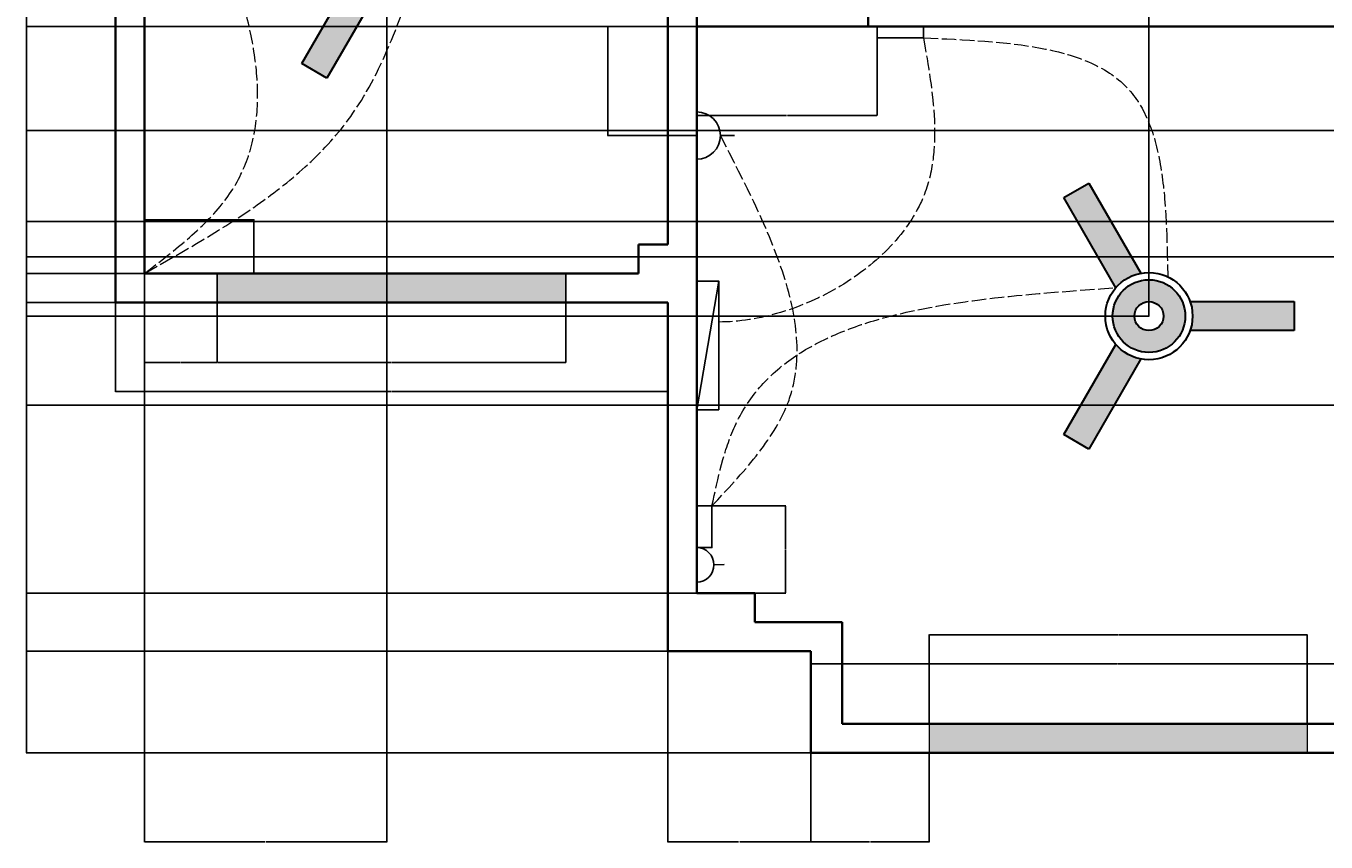
# Model space of a CAD drawing. Units: inches. Extents: x 2034 to 3646, y 962 to 2549.
# Tile 1 of 4: x 2034 to 3108, y 962 to 1636. Entities that reach past the tile are written whole.
import ezdxf

# ---------------------------------------------------------------- set-up
doc = ezdxf.new("R2010")
doc.units = ezdxf.units.IN
doc.linetypes.add('ACAD_ISO02W100', pattern=[15, 12, -3])
for name, color, linetype, lineweight in [('A-ANNO-DIMS', 2, 'Continuous', 18), ('A-GLAZ', 250, 'Continuous', 18), ('E-EQPM-FANS', 7, 'Continuous', 30), ('E-LITE-CTRL', 7, 'Continuous', 25), ('E-LITE-FIXT', 7, 'Continuous', 25), ('E-POWR-DEVC', 7, 'Continuous', 25)]:
    doc.layers.add(name, color=color, linetype=linetype, lineweight=lineweight)
for name, color, linetype, lineweight, true_color in [('A-GLAZ-PATT', 18, 'Continuous', 13, 0x000000), ('A-WALL', 203, 'Continuous', 35, 0xa780c2), ('E-LITE-WIRE', 103, 'ACAD_ISO02W100', 18, 0x6dc08b)]:
    doc.layers.add(name, color=color, linetype=linetype, lineweight=lineweight, true_color=true_color)
doc.styles.get("Standard").update_dxf_attribs({"font": 'arial.ttf'})
doc.dimstyles.get("Standard").update_dxf_attribs({"dimtxt": 0.18, "dimasz": 0.18, "dimexe": 0.18, "dimexo": 0.0625, "dimgap": 0.09, "dimtad": 0, "dimtih": 1, "dimtoh": 1, "dimdec": 4, "dimzin": 0, "dimdsep": 46, "dimtxsty": 'Standard', "dimcen": 0.09, "dimadec": 0, "dimazin": 0, "dimtfac": 1, "dimtdec": 4, "dimtofl": 0, "dimtmove": 0, "dimatfit": 3, "dimfxl": 1, "dimtolj": 1, "dimtzin": 0, "dimarcsym": 0})

# ---------------------------------------------------------------- blocks, each defined once
blk = doc.blocks.new('CEILING-FAN-3-BLADE')
h = blk.add_hatch(color=256)
h.dxf.hatch_style = 1
h.paths.add_polyline_path([(-49.6, 109.9), (-70.4, 97.9), (-27.4, 23.4, -0.171573), (-6.6, 35.4)])
h = blk.add_hatch(color=256)
h.dxf.hatch_style = 1
h.paths.add_polyline_path([(-30, 0, 1), (30, 0, 1)])
h.paths.add_polyline_path([(12, 0, -1), (-12, 0, -1)], flags=16)
h = blk.add_hatch(color=256)
h.dxf.hatch_style = 1
h.paths.add_polyline_path([(120, 12), (33.9, 12, -0.085164), (36, 0, -0.085164), (33.9, -12), (120, -12)])
h = blk.add_hatch(color=256)
h.dxf.hatch_style = 1
h.paths.add_polyline_path([(-6.6, -35.4, -0.171573), (-27.4, -23.4), (-70.4, -97.9), (-49.6, -109.9)])
for p, q in [((-70.4, 97.9), (-49.6, 109.9)), ((-49.6, 109.9), (-6.6, 35.4)), ((-27.4, 23.4), (-70.4, 97.9)), ((33.9, 12), (120, 12)), ((120, 12), (120, -12)), ((120, -12), (33.9, -12)), ((-70.4, -97.9), (-27.4, -23.4)), ((-6.6, -35.4), (-49.6, -109.9)), ((-49.6, -109.9), (-70.4, -97.9))]:
    blk.add_line(p, q)
for radius in [36, 30, 12]:
    blk.add_circle((0, 0), radius)
blk = doc.blocks.new('*D5')
at = {"layer": 'A-ANNO-DIMS', "color": 0, "lineweight": -2, "transparency": 16777216}
for p, q in [((2108.1, 2475.6), (2034.6, 2475.6)), ((2034.7, 2475.5), (2034.7, 1755.8)), ((2034.7, 1035.8), (2034.7, 1755.5)), ((2682.3, 1035.6), (2034.6, 1035.6))]:
    blk.add_line(p, q, dxfattribs=at)
at = {"layer": 'A-ANNO-DIMS', "color": 0, "transparency": 16777216}
for points in [[(2034.7, 2475.5), (2034.8, 2475.5), (2034.7, 2475.6)], [(2034.7, 1035.8), (2034.8, 1035.8), (2034.7, 1035.6)]]:
    blk.add_solid(points, dxfattribs=at)
at = {"layer": 'Defpoints', "color": 0, "transparency": 16777216}
for p in [(2034.7, 2475.6), (2108.2, 2475.6), (2682.3, 1035.6)]:
    blk.add_point(p, dxfattribs=at)
at = {"layer": 'A-ANNO-DIMS', "color": 0, "transparency": 16777216, "insert": (2034.7, 1755.6), "char_height": 0.18, "attachment_point": 5}
blk.add_mtext('\\A1;1440', dxfattribs=at)
blk = doc.blocks.new('*D6')
at = {"layer": 'A-ANNO-DIMS', "color": 0, "lineweight": -2, "transparency": 16777216}
for p, q in [((2108.2, 1407.6), (2108.2, 1334)), ((2564.2, 1407.6), (2564.2, 1334)), ((2108.4, 1334.2), (2335.9, 1334.2)), ((2564, 1334.2), (2336.5, 1334.2))]:
    blk.add_line(p, q, dxfattribs=at)
at = {"layer": 'A-ANNO-DIMS', "color": 0, "transparency": 16777216}
for points in [[(2108.4, 1334.2), (2108.4, 1334.2), (2108.2, 1334.2)], [(2564, 1334.2), (2564, 1334.2), (2564.2, 1334.2)]]:
    blk.add_solid(points, dxfattribs=at)
at = {"layer": 'Defpoints', "color": 0, "transparency": 16777216}
for p in [(2108.2, 1407.6), (2564.2, 1407.6), (2108.2, 1334.2)]:
    blk.add_point(p, dxfattribs=at)
at = {"layer": 'A-ANNO-DIMS', "color": 0, "transparency": 16777216, "insert": (2336.2, 1334.2), "char_height": 0.18, "attachment_point": 5}
blk.add_mtext('\\A1;456', dxfattribs=at)
blk = doc.blocks.new('*D7')
at = {"layer": 'A-ANNO-DIMS', "color": 0, "lineweight": -2, "transparency": 16777216}
for p, q in [((2564.2, 1119.6), (2564.2, 962)), ((2682.3, 1119.6), (2682.3, 962)), ((2564.4, 962.2), (2622.8, 962.2)), ((2682.1, 962.2), (2623.7, 962.2))]:
    blk.add_line(p, q, dxfattribs=at)
at = {"layer": 'A-ANNO-DIMS', "color": 0, "transparency": 16777216}
for points in [[(2564.4, 962.2), (2564.4, 962.2), (2564.2, 962.2)], [(2682.1, 962.2), (2682.1, 962.2), (2682.3, 962.2)]]:
    blk.add_solid(points, dxfattribs=at)
at = {"layer": 'Defpoints', "color": 0, "transparency": 16777216}
for p in [(2564.2, 1119.6), (2682.3, 1119.6), (2682.3, 962.2)]:
    blk.add_point(p, dxfattribs=at)
at = {"layer": 'A-ANNO-DIMS', "color": 0, "transparency": 16777216, "insert": (2623.3, 962.2), "char_height": 0.18, "attachment_point": 5}
blk.add_mtext('\\A1;118.12', dxfattribs=at)
blk = doc.blocks.new('*D8')
at = {"layer": 'A-ANNO-DIMS', "color": 0, "lineweight": -2, "transparency": 16777216}
for p, q in [((2682.3, 1035.7), (2682.3, 1109.3)), ((2682.5, 1109.1), (2935.5, 1109.1)), ((3189.4, 1109.1), (2936.3, 1109.1)), ((3189.6, 1035.7), (3189.6, 1109.3))]:
    blk.add_line(p, q, dxfattribs=at)
at = {"layer": 'A-ANNO-DIMS', "color": 0, "transparency": 16777216}
for points in [[(2682.5, 1109.1), (2682.5, 1109.1), (2682.3, 1109.1)], [(3189.4, 1109.1), (3189.4, 1109.1), (3189.6, 1109.1)]]:
    blk.add_solid(points, dxfattribs=at)
at = {"layer": 'Defpoints', "color": 0, "transparency": 16777216}
for p in [(3189.6, 1109.1), (2682.3, 1035.6), (3189.6, 1035.6)]:
    blk.add_point(p, dxfattribs=at)
at = {"layer": 'A-ANNO-DIMS', "color": 0, "transparency": 16777216, "insert": (2935.9, 1109.1), "char_height": 0.18, "attachment_point": 5}
blk.add_mtext('\\A1;507.2', dxfattribs=at)
blk = doc.blocks.new('*D9')
at = {"layer": 'A-ANNO-DIMS', "color": 0, "lineweight": -2, "transparency": 16777216}
for p, q in [((2564.1, 1407.6), (2034.6, 1407.6)), ((2034.7, 1407.5), (2034.7, 1263.8)), ((2034.7, 1119.8), (2034.7, 1263.5)), ((2564.1, 1119.6), (2034.6, 1119.6))]:
    blk.add_line(p, q, dxfattribs=at)
at = {"layer": 'A-ANNO-DIMS', "color": 0, "transparency": 16777216}
for points in [[(2034.7, 1407.5), (2034.8, 1407.5), (2034.7, 1407.6)], [(2034.7, 1119.8), (2034.8, 1119.8), (2034.7, 1119.6)]]:
    blk.add_solid(points, dxfattribs=at)
at = {"layer": 'Defpoints', "color": 0, "transparency": 16777216}
for p in [(2034.7, 1407.6), (2564.2, 1407.6), (2564.2, 1119.6)]:
    blk.add_point(p, dxfattribs=at)
at = {"layer": 'A-ANNO-DIMS', "color": 0, "transparency": 16777216, "insert": (2034.7, 1263.6), "char_height": 0.18, "attachment_point": 5}
blk.add_mtext('\\A1;288', dxfattribs=at)
blk = doc.blocks.new('*D10')
at = {"layer": 'A-ANNO-DIMS', "color": 0, "lineweight": -2, "transparency": 16777216}
for p, q in [((2682.3, 1119.6), (2034.6, 1119.6)), ((2034.7, 1119.5), (2034.7, 1077.8)), ((2034.7, 1035.8), (2034.7, 1077.5)), ((2682.3, 1035.6), (2034.6, 1035.6))]:
    blk.add_line(p, q, dxfattribs=at)
at = {"layer": 'A-ANNO-DIMS', "color": 0, "transparency": 16777216}
for points in [[(2034.7, 1119.5), (2034.8, 1119.5), (2034.7, 1119.6)], [(2034.7, 1035.8), (2034.8, 1035.8), (2034.7, 1035.6)]]:
    blk.add_solid(points, dxfattribs=at)
at = {"layer": 'Defpoints', "color": 0, "transparency": 16777216}
for p in [(2034.7, 1119.6), (2682.3, 1119.6), (2682.3, 1035.6)]:
    blk.add_point(p, dxfattribs=at)
at = {"layer": 'A-ANNO-DIMS', "color": 0, "transparency": 16777216, "insert": (2034.7, 1077.6), "char_height": 0.18, "attachment_point": 5}
blk.add_mtext('\\A1;84', dxfattribs=at)
blk = doc.blocks.new('*D16')
at = {"layer": 'A-ANNO-DIMS', "color": 0, "lineweight": -2, "transparency": 16777216}
for p, q in [((2588.2, 1635.7), (2588.2, 2549.3)), ((2588.4, 2549.1), (2935.9, 2549.1)), ((3284, 2549.1), (2936.5, 2549.1)), ((3284.2, 1635.7), (3284.2, 2549.3))]:
    blk.add_line(p, q, dxfattribs=at)
at = {"layer": 'A-ANNO-DIMS', "color": 0, "transparency": 16777216}
for points in [[(2588.4, 2549.1), (2588.4, 2549.1), (2588.2, 2549.1)], [(3284, 2549.1), (3284, 2549.1), (3284.2, 2549.1)]]:
    blk.add_solid(points, dxfattribs=at)
at = {"layer": 'Defpoints', "color": 0, "transparency": 16777216}
for p in [(3284.2, 2549.1), (2588.2, 1635.6), (3284.2, 1635.6)]:
    blk.add_point(p, dxfattribs=at)
at = {"layer": 'A-ANNO-DIMS', "color": 0, "transparency": 16777216, "insert": (2936.2, 2549.1), "char_height": 0.18, "attachment_point": 5}
blk.add_mtext('\\A1;696', dxfattribs=at)
blk = doc.blocks.new('*D17')
at = {"layer": 'A-ANNO-DIMS', "color": 0, "lineweight": -2, "transparency": 16777216}
for p, q in [((2588.1, 1635.6), (2034.6, 1635.6)), ((2034.7, 1635.5), (2034.7, 1401.8)), ((2034.7, 1167.8), (2034.7, 1401.5)), ((2588.1, 1167.6), (2034.6, 1167.6))]:
    blk.add_line(p, q, dxfattribs=at)
at = {"layer": 'A-ANNO-DIMS', "color": 0, "transparency": 16777216}
for points in [[(2034.7, 1635.5), (2034.8, 1635.5), (2034.7, 1635.6)], [(2034.7, 1167.8), (2034.8, 1167.8), (2034.7, 1167.6)]]:
    blk.add_solid(points, dxfattribs=at)
at = {"layer": 'Defpoints', "color": 0, "transparency": 16777216}
for p in [(2034.7, 1635.6), (2588.2, 1635.6), (2588.2, 1167.6)]:
    blk.add_point(p, dxfattribs=at)
at = {"layer": 'A-ANNO-DIMS', "color": 0, "transparency": 16777216, "insert": (2034.7, 1401.6), "char_height": 0.18, "attachment_point": 5}
blk.add_mtext('\\A1;468', dxfattribs=at)
blk = doc.blocks.new('*D30')
at = {"layer": 'A-ANNO-DIMS', "color": 0, "lineweight": -2, "transparency": 16777216}
for p, q in [((2332.4, 1702.8), (2332.4, 962)), ((2132.2, 1431.6), (2132.2, 962)), ((2132.4, 962.2), (2231.9, 962.2)), ((2332.3, 962.2), (2232.8, 962.2))]:
    blk.add_line(p, q, dxfattribs=at)
at = {"layer": 'A-ANNO-DIMS', "color": 0, "transparency": 16777216}
for points in [[(2132.4, 962.2), (2132.4, 962.2), (2132.2, 962.2)], [(2332.3, 962.2), (2332.3, 962.2), (2332.4, 962.2)]]:
    blk.add_solid(points, dxfattribs=at)
at = {"layer": 'Defpoints', "color": 0, "transparency": 16777216}
for p in [(2332.4, 1702.9), (2132.2, 1431.6), (2332.4, 962.2)]:
    blk.add_point(p, dxfattribs=at)
at = {"layer": 'A-ANNO-DIMS', "color": 0, "transparency": 16777216, "insert": (2232.3, 962.2), "char_height": 0.18, "attachment_point": 5}
blk.add_mtext('\\A1;200.24', dxfattribs=at)
blk = doc.blocks.new('*D31')
at = {"layer": 'A-ANNO-DIMS', "color": 0, "lineweight": -2, "transparency": 16777216}
for p, q in [((2332.4, 1702.9), (2034.6, 1702.9)), ((2034.7, 1702.7), (2034.7, 1567.4)), ((2034.7, 1431.8), (2034.7, 1567.1)), ((2132.1, 1431.6), (2034.6, 1431.6))]:
    blk.add_line(p, q, dxfattribs=at)
at = {"layer": 'A-ANNO-DIMS', "color": 0, "transparency": 16777216}
for points in [[(2034.7, 1702.7), (2034.8, 1702.7), (2034.7, 1702.9)], [(2034.7, 1431.8), (2034.8, 1431.8), (2034.7, 1431.6)]]:
    blk.add_solid(points, dxfattribs=at)
at = {"layer": 'Defpoints', "color": 0, "transparency": 16777216}
for p in [(2034.7, 1702.9), (2332.4, 1702.9), (2132.2, 1431.6)]:
    blk.add_point(p, dxfattribs=at)
at = {"layer": 'A-ANNO-DIMS', "color": 0, "transparency": 16777216, "insert": (2034.7, 1567.3), "char_height": 0.18, "attachment_point": 5}
blk.add_mtext('\\A1;271.24', dxfattribs=at)
blk = doc.blocks.new('*D33')
at = {"layer": 'A-ANNO-DIMS', "color": 0, "lineweight": -2, "transparency": 16777216}
for p, q in [((2961.6, 1396.5), (2961.6, 2549.3)), ((2961.8, 2549.1), (3122.5, 2549.1)), ((3284, 2549.1), (3123.3, 2549.1)), ((3284.2, 1305), (3284.2, 2549.3))]:
    blk.add_line(p, q, dxfattribs=at)
at = {"layer": 'A-ANNO-DIMS', "color": 0, "transparency": 16777216}
for points in [[(2961.8, 2549.1), (2961.8, 2549.1), (2961.6, 2549.1)], [(3284, 2549.1), (3284, 2549.1), (3284.2, 2549.1)]]:
    blk.add_solid(points, dxfattribs=at)
at = {"layer": 'Defpoints', "color": 0, "transparency": 16777216}
for p in [(3284.2, 2549.1), (2961.6, 1396.4), (3284.2, 1304.9)]:
    blk.add_point(p, dxfattribs=at)
at = {"layer": 'A-ANNO-DIMS', "color": 0, "transparency": 16777216, "insert": (3122.9, 2549.1), "char_height": 0.18, "attachment_point": 5}
blk.add_mtext('\\A1;322.6', dxfattribs=at)
blk = doc.blocks.new('*D34')
at = {"layer": 'A-ANNO-DIMS', "color": 0, "lineweight": -2, "transparency": 16777216}
for p, q in [((2737.1, 1635.6), (2034.6, 1635.6)), ((2034.7, 1635.5), (2034.7, 1516.2)), ((2034.7, 1396.6), (2034.7, 1515.9)), ((2961.5, 1396.4), (2034.6, 1396.4))]:
    blk.add_line(p, q, dxfattribs=at)
at = {"layer": 'A-ANNO-DIMS', "color": 0, "transparency": 16777216}
for points in [[(2034.7, 1635.5), (2034.8, 1635.5), (2034.7, 1635.6)], [(2034.7, 1396.6), (2034.8, 1396.6), (2034.7, 1396.4)]]:
    blk.add_solid(points, dxfattribs=at)
at = {"layer": 'Defpoints', "color": 0, "transparency": 16777216}
for p in [(2034.7, 1635.6), (2737.2, 1635.6), (2961.6, 1396.4)]:
    blk.add_point(p, dxfattribs=at)
at = {"layer": 'A-ANNO-DIMS', "color": 0, "transparency": 16777216, "insert": (2034.7, 1516), "char_height": 0.18, "attachment_point": 5}
blk.add_mtext('\\A1;239.2', dxfattribs=at)
blk = doc.blocks.new('*D35')
at = {"layer": 'A-ANNO-DIMS', "color": 0, "lineweight": -2, "transparency": 16777216}
for p, q in [((2132.2, 1431.6), (2132.2, 1358)), ((2192.2, 1431.6), (2192.2, 1358)), ((2132.4, 1358.2), (2162, 1358.2)), ((2192, 1358.2), (2162.4, 1358.2))]:
    blk.add_line(p, q, dxfattribs=at)
at = {"layer": 'A-ANNO-DIMS', "color": 0, "transparency": 16777216}
for points in [[(2132.4, 1358.2), (2132.4, 1358.2), (2132.2, 1358.2)], [(2192, 1358.2), (2192, 1358.2), (2192.2, 1358.2)]]:
    blk.add_solid(points, dxfattribs=at)
at = {"layer": 'Defpoints', "color": 0, "transparency": 16777216}
for p in [(2132.2, 1431.6), (2192.2, 1431.6), (2132.2, 1358.2)]:
    blk.add_point(p, dxfattribs=at)
at = {"layer": 'A-ANNO-DIMS', "color": 0, "transparency": 16777216, "insert": (2162.2, 1358.2), "char_height": 0.18, "attachment_point": 5}
blk.add_mtext('\\A1;60', dxfattribs=at)
blk = doc.blocks.new('*D36')
at = {"layer": 'A-ANNO-DIMS', "color": 0, "lineweight": -2, "transparency": 16777216}
for p, q in [((2192.2, 1431.6), (2192.2, 1358)), ((2480.2, 1431.6), (2480.2, 1358)), ((2192.4, 1358.2), (2335.9, 1358.2)), ((2480, 1358.2), (2336.5, 1358.2))]:
    blk.add_line(p, q, dxfattribs=at)
at = {"layer": 'A-ANNO-DIMS', "color": 0, "transparency": 16777216}
for points in [[(2192.4, 1358.2), (2192.4, 1358.2), (2192.2, 1358.2)], [(2480, 1358.2), (2480, 1358.2), (2480.2, 1358.2)]]:
    blk.add_solid(points, dxfattribs=at)
at = {"layer": 'Defpoints', "color": 0, "transparency": 16777216}
for p in [(2192.2, 1431.6), (2480.2, 1431.6), (2192.2, 1358.2)]:
    blk.add_point(p, dxfattribs=at)
at = {"layer": 'A-ANNO-DIMS', "color": 0, "transparency": 16777216, "insert": (2336.2, 1358.2), "char_height": 0.18, "attachment_point": 5}
blk.add_mtext('\\A1;288', dxfattribs=at)
blk = doc.blocks.new('*D37')
at = {"layer": 'A-ANNO-DIMS', "color": 0, "lineweight": -2, "transparency": 16777216}
for p, q in [((2682.3, 1035.6), (2682.3, 962)), ((2780.2, 1035.6), (2780.2, 962)), ((2682.5, 962.2), (2730.9, 962.2)), ((2780, 962.2), (2731.7, 962.2))]:
    blk.add_line(p, q, dxfattribs=at)
at = {"layer": 'A-ANNO-DIMS', "color": 0, "transparency": 16777216}
for points in [[(2682.5, 962.2), (2682.5, 962.2), (2682.3, 962.2)], [(2780, 962.2), (2780, 962.2), (2780.2, 962.2)]]:
    blk.add_solid(points, dxfattribs=at)
at = {"layer": 'Defpoints', "color": 0, "transparency": 16777216}
for p in [(2682.3, 1035.6), (2780.2, 1035.6), (2780.2, 962.2)]:
    blk.add_point(p, dxfattribs=at)
at = {"layer": 'A-ANNO-DIMS', "color": 0, "transparency": 16777216, "insert": (2731.3, 962.2), "char_height": 0.18, "attachment_point": 5}
blk.add_mtext('\\A1;97.88', dxfattribs=at)
blk = doc.blocks.new('*D38')
at = {"layer": 'A-ANNO-DIMS', "color": 0, "lineweight": -2, "transparency": 16777216}
for p, q in [((2780.2, 1059.7), (2780.2, 1133.3)), ((2780.4, 1133.1), (2935.9, 1133.1)), ((3092, 1133.1), (2936.5, 1133.1)), ((3092.2, 1059.7), (3092.2, 1133.3))]:
    blk.add_line(p, q, dxfattribs=at)
at = {"layer": 'A-ANNO-DIMS', "color": 0, "transparency": 16777216}
for points in [[(2780.4, 1133.1), (2780.4, 1133.1), (2780.2, 1133.1)], [(3092, 1133.1), (3092, 1133.1), (3092.2, 1133.1)]]:
    blk.add_solid(points, dxfattribs=at)
at = {"layer": 'Defpoints', "color": 0, "transparency": 16777216}
for p in [(3092.2, 1133.1), (2780.2, 1059.6), (3092.2, 1059.6)]:
    blk.add_point(p, dxfattribs=at)
at = {"layer": 'A-ANNO-DIMS', "color": 0, "transparency": 16777216, "insert": (2936.2, 1133.1), "char_height": 0.18, "attachment_point": 5}
blk.add_mtext('\\A1;312', dxfattribs=at)
blk = doc.blocks.new('*D49')
at = {"layer": 'A-ANNO-DIMS', "color": 0, "lineweight": -2, "transparency": 16777216}
for p, q in [((3392.3, 1474.6), (2034.6, 1474.6)), ((2034.7, 1474.4), (2034.7, 1398.9)), ((2034.7, 1323), (2034.7, 1398.5)), ((3392.3, 1322.8), (2034.6, 1322.8))]:
    blk.add_line(p, q, dxfattribs=at)
at = {"layer": 'A-ANNO-DIMS', "color": 0, "transparency": 16777216}
for points in [[(2034.7, 1474.4), (2034.8, 1474.4), (2034.7, 1474.6)], [(2034.7, 1323), (2034.8, 1323), (2034.7, 1322.8)]]:
    blk.add_solid(points, dxfattribs=at)
at = {"layer": 'Defpoints', "color": 0, "transparency": 16777216}
for p in [(2034.7, 1474.6), (3392.3, 1474.6), (3392.3, 1322.8)]:
    blk.add_point(p, dxfattribs=at)
at = {"layer": 'A-ANNO-DIMS', "color": 0, "transparency": 16777216, "insert": (2034.7, 1398.7), "char_height": 0.18, "attachment_point": 5}
blk.add_mtext('\\A1;151.76', dxfattribs=at)
blk = doc.blocks.new('*D52')
at = {"layer": 'A-ANNO-DIMS', "color": 0, "lineweight": -2, "transparency": 16777216}
for p, q in [((3284.1, 1549.7), (2034.6, 1549.7)), ((2034.7, 1549.5), (2034.7, 1497.7)), ((2034.7, 1445.5), (2034.7, 1497.3)), ((3284.1, 1445.3), (2034.6, 1445.3))]:
    blk.add_line(p, q, dxfattribs=at)
at = {"layer": 'A-ANNO-DIMS', "color": 0, "transparency": 16777216}
for points in [[(2034.7, 1549.5), (2034.8, 1549.5), (2034.7, 1549.7)], [(2034.7, 1445.5), (2034.8, 1445.5), (2034.7, 1445.3)]]:
    blk.add_solid(points, dxfattribs=at)
at = {"layer": 'Defpoints', "color": 0, "transparency": 16777216}
for p in [(2034.7, 1549.7), (3284.2, 1549.7), (3284.2, 1445.3)]:
    blk.add_point(p, dxfattribs=at)
at = {"layer": 'A-ANNO-DIMS', "color": 0, "transparency": 16777216, "insert": (2034.7, 1497.5), "char_height": 0.18, "attachment_point": 5}
blk.add_mtext('\\A1;104.39', dxfattribs=at)
blk = doc.blocks.new('*D54')
at = {"layer": 'A-ANNO-DIMS', "color": 0, "lineweight": -2, "transparency": 16777216}
for p, q in [((2588.2, 1635.6), (2588.2, 1562)), ((2737.2, 1635.6), (2737.2, 1562)), ((2588.4, 1562.2), (2662.2, 1562.2)), ((2737, 1562.2), (2663.1, 1562.2))]:
    blk.add_line(p, q, dxfattribs=at)
at = {"layer": 'A-ANNO-DIMS', "color": 0, "transparency": 16777216}
for points in [[(2588.4, 1562.2), (2588.4, 1562.2), (2588.2, 1562.2)], [(2737, 1562.2), (2737, 1562.2), (2737.2, 1562.2)]]:
    blk.add_solid(points, dxfattribs=at)
at = {"layer": 'Defpoints', "color": 0, "transparency": 16777216}
for p in [(2588.2, 1635.6), (2737.2, 1635.6), (2588.2, 1562.2)]:
    blk.add_point(p, dxfattribs=at)
at = {"layer": 'A-ANNO-DIMS', "color": 0, "transparency": 16777216, "insert": (2662.7, 1562.2), "char_height": 0.18, "attachment_point": 5}
blk.add_mtext('\\A1;148.97', dxfattribs=at)
blk = doc.blocks.new('*D58')
at = {"layer": 'A-ANNO-DIMS', "color": 0, "lineweight": -2, "transparency": 16777216}
for p, q in [((2588.1, 1635.6), (2514.6, 1635.6)), ((2514.7, 1635.5), (2514.7, 1590.8)), ((2514.7, 1545.7), (2514.7, 1590.4)), ((2588.1, 1545.5), (2514.6, 1545.5))]:
    blk.add_line(p, q, dxfattribs=at)
at = {"layer": 'A-ANNO-DIMS', "color": 0, "transparency": 16777216}
for points in [[(2514.7, 1635.5), (2514.8, 1635.5), (2514.7, 1635.6)], [(2514.7, 1545.7), (2514.8, 1545.7), (2514.7, 1545.5)]]:
    blk.add_solid(points, dxfattribs=at)
at = {"layer": 'Defpoints', "color": 0, "transparency": 16777216}
for p in [(2514.7, 1635.6), (2588.2, 1635.6), (2588.2, 1545.5)]:
    blk.add_point(p, dxfattribs=at)
at = {"layer": 'A-ANNO-DIMS', "color": 0, "transparency": 16777216, "insert": (2514.7, 1590.6), "char_height": 0.18, "attachment_point": 5}
blk.add_mtext('\\A1;90.1', dxfattribs=at)
blk = doc.blocks.new('*D60')
at = {"layer": 'A-ANNO-DIMS', "color": 0, "lineweight": -2, "transparency": 16777216}
for p, q in [((2588.3, 1239.6), (2661.8, 1239.6)), ((2661.6, 1239.4), (2661.6, 1203.8)), ((2661.6, 1167.8), (2661.6, 1203.4)), ((2588.3, 1167.6), (2661.8, 1167.6))]:
    blk.add_line(p, q, dxfattribs=at)
at = {"layer": 'A-ANNO-DIMS', "color": 0, "transparency": 16777216}
for points in [[(2661.6, 1239.4), (2661.7, 1239.4), (2661.6, 1239.6)], [(2661.6, 1167.8), (2661.7, 1167.8), (2661.6, 1167.6)]]:
    blk.add_solid(points, dxfattribs=at)
at = {"layer": 'Defpoints', "color": 0, "transparency": 16777216}
for p in [(2588.2, 1239.6), (2588.2, 1167.6), (2661.6, 1167.6)]:
    blk.add_point(p, dxfattribs=at)
at = {"layer": 'A-ANNO-DIMS', "color": 0, "transparency": 16777216, "insert": (2661.6, 1203.6), "char_height": 0.18, "attachment_point": 5}
blk.add_mtext('\\A1;71.98', dxfattribs=at)
blk = doc.blocks.new('*D64')
at = {"layer": 'A-ANNO-DIMS', "color": 0, "lineweight": -2, "transparency": 16777216}
for p, q in [((2904, 1396.4), (2925.4, 1396.4)), ((2961.5, 1396.4), (2961.7, 1396.4)), ((2961.6, 1396.3), (2961.6, 1396.5))]:
    blk.add_line(p, q, dxfattribs=at)
at = {"layer": 'A-ANNO-DIMS', "color": 0, "transparency": 16777216}
blk.add_solid([(2925.4, 1396.5), (2925.4, 1396.4), (2925.6, 1396.4)], dxfattribs=at)
at = {"layer": 'Defpoints', "color": 0, "transparency": 16777216}
for p in [(2925.6, 1396.4), (2997.6, 1396.4)]:
    blk.add_point(p, dxfattribs=at)
at = {"layer": 'A-ANNO-DIMS', "color": 0, "transparency": 16777216, "insert": (2903.5, 1396.4), "char_height": 0.18, "attachment_point": 5}
blk.add_mtext('\\A1;4X ∅72', dxfattribs=at)
blk = doc.blocks.new('*D72')
at = {"layer": 'A-ANNO-DIMS', "color": 0, "lineweight": -2, "transparency": 16777216}
for p, q in [((2588.1, 1545.5), (2588.3, 1545.5)), ((2588.2, 1545.4), (2588.2, 1545.6)), ((2619.4, 1545.5), (2607.9, 1545.5))]:
    blk.add_line(p, q, dxfattribs=at)
at = {"layer": 'A-ANNO-DIMS', "color": 0, "transparency": 16777216}
blk.add_solid([(2607.9, 1545.6), (2607.9, 1545.5), (2607.7, 1545.5)], dxfattribs=at)
at = {"layer": 'Defpoints', "color": 0, "transparency": 16777216}
for p in [(2588.2, 1545.5), (2607.7, 1545.5)]:
    blk.add_point(p, dxfattribs=at)
at = {"layer": 'A-ANNO-DIMS', "color": 0, "transparency": 16777216, "insert": (2620, 1545.5), "char_height": 0.18, "attachment_point": 5}
blk.add_mtext('\\A1;R19.526', dxfattribs=at)
blk = doc.blocks.new('*D78')
at = {"layer": 'A-ANNO-DIMS', "color": 0, "lineweight": -2, "transparency": 16777216}
for p, q in [((2588.1, 1190.9), (2588.3, 1190.9)), ((2588.2, 1190.9), (2588.2, 1191)), ((2610.9, 1191.2), (2602.6, 1191.1))]:
    blk.add_line(p, q, dxfattribs=at)
at = {"layer": 'A-ANNO-DIMS', "color": 0, "transparency": 16777216}
blk.add_solid([(2602.6, 1191.1), (2602.6, 1191.1), (2602.4, 1191.1)], dxfattribs=at)
at = {"layer": 'Defpoints', "color": 0, "transparency": 16777216}
for p in [(2588.2, 1190.9), (2602.4, 1191.1)]:
    blk.add_point(p, dxfattribs=at)
at = {"layer": 'A-ANNO-DIMS', "color": 0, "transparency": 16777216, "insert": (2611.4, 1191.2), "char_height": 0.18, "attachment_point": 5}
blk.add_mtext('\\A1;R14.22', dxfattribs=at)

msp = doc.modelspace()

# ---------------------------------------------------------------- hatches: boundary and pattern name
at = {"layer": 'A-GLAZ-PATT'}
h = msp.add_hatch(color=256, dxfattribs=at)
h.dxf.hatch_style = 1
h.paths.add_polyline_path([(2480.1976, 1431.6388), (2192.1976, 1431.6388), (2192.1976, 1407.6388), (2480.1976, 1407.6388)])
h = msp.add_hatch(color=256, dxfattribs=at)
h.dxf.hatch_style = 1
h.paths.add_polyline_path([(3092.1976, 1059.6388), (2780.1976, 1059.6388), (2780.1976, 1035.6388), (3092.1976, 1035.6388)])

# ---------------------------------------------------------------- linework, layer by layer
at = {"layer": 'A-GLAZ'}
for p, q in [((2192.1976, 1431.6388), (2192.1976, 1407.6388)), ((2192.1976, 1431.6388), (2480.1976, 1431.6388)), ((2480.1976, 1431.6388), (2480.1976, 1407.6388)), ((2192.1976, 1407.6388), (2480.1976, 1407.6388)), ((2780.1976, 1059.6388), (2780.1976, 1035.6388)), ((2780.1976, 1059.6388), (3092.1976, 1059.6388)), ((3092.1976, 1059.6388), (3092.1976, 1035.6388)), ((2780.1976, 1035.6388), (3092.1976, 1035.6388))]:
    msp.add_line(p, q, dxfattribs=at)
at = {"layer": 'A-WALL'}
for p, q in [((2588.1976, 1167.6388), (2588.1976, 1971.6388)), ((2132.1976, 1431.6388), (2132.1976, 1947.6388)), ((2564.1976, 1455.6388), (2564.1976, 1875.6388)), ((2729.8258, 1659.6388), (2729.8258, 1635.6388)), ((2588.1976, 1635.6388), (3284.1976, 1635.6388)), ((2540.1976, 1431.6388), (2540.1976, 1455.6388)), ((2540.1976, 1455.6388), (2564.1976, 1455.6388)), ((2132.1976, 1431.6388), (2540.1976, 1431.6388)), ((2132.1976, 1407.6388), (2108.1976, 1407.6388)), ((2132.1976, 1407.6388), (2564.1976, 1407.6388)), ((2564.1976, 1119.6388), (2564.1976, 1407.6388)), ((2636.1976, 1167.6388), (2588.1976, 1167.6388)), ((2636.1976, 1143.6388), (2636.1976, 1167.6388)), ((2708.1976, 1143.6388), (2636.1976, 1143.6388)), ((2708.1976, 1059.6388), (2708.1976, 1143.6388)), ((2682.3208, 1119.6388), (2564.1976, 1119.6388)), ((2682.3208, 1035.6388), (2682.3208, 1119.6388)), ((3164.1976, 1059.6388), (2708.1976, 1059.6388)), ((3189.5638, 1035.6388), (2682.3208, 1035.6388)), ((2706.3208, 1035.6388), (2682.3208, 1035.6388))]:
    msp.add_line(p, q, dxfattribs=at)
msp.add_lwpolyline([(2108.1976, 1407.6388), (2108.1976, 2475.6388), (3308.1976, 2475.6388)], dxfattribs=at)
at = {"layer": 'E-LITE-CTRL'}
for points in [[(2737.172, 1635.6388), (2775.458, 1635.6388), (2775.458, 1626.2502), (2737.172, 1626.2502)], [(2132.1976, 1431.6388), (2222.5717, 1431.6388), (2222.5717, 1476.0422), (2132.1976, 1476.0422)], [(2588.1976, 1205.1613), (2600.7258, 1205.1613), (2600.7258, 1239.6163), (2588.1976, 1239.6163)]]:
    msp.add_lwpolyline(points, close=True, dxfattribs=at)
at = {"layer": 'E-LITE-FIXT'}
msp.add_line((2606.4152, 1425.3903), (2588.1976, 1319.1329), dxfattribs=at)
msp.add_lwpolyline([(2588.1976, 1425.3903), (2606.4152, 1425.3903), (2606.4152, 1319.1329), (2588.1976, 1319.1329)], close=True, dxfattribs=at)
at = {"layer": 'E-LITE-WIRE'}
for points, knots in [([(2132.1976, 1431.6388), (2157.638, 1451.201), (2276.6339, 1542.7023), (2202.4164, 1700.7955), (2144.0659, 1825.0897)], [0, 0, 0, 0, 91.463199701, 427.814592014, 427.814592014, 427.814592014, 427.814592014]), ([(2132.1976, 1431.6388), (2198.2305, 1468.9918), (2306.37, 1530.1634), (2344.9098, 1645.8124), (2359.9161, 1690.843)], [0, 0, 0, 0, 217.156530493, 355.629044919, 355.629044919, 355.629044919, 355.629044919]), ([(2775.458, 1626.2502), (2783.4011, 1580.4234), (2803.3836, 1465.1371), (2672.4325, 1391.5072), (2606.2065, 1391.5305), (2606.1022, 1391.5306)], [0, 0, 0, 0, 130.887293215, 329.272351587, 329.58530176, 329.58530176, 329.58530176, 329.58530176]), ([(2775.458, 1626.2502), (2843.6443, 1623.2777), (2973.5056, 1617.6165), (2975.9452, 1489.6758), (2977.1038, 1428.9129)], [0, 0, 0, 0, 174.709563386, 332.73592807, 332.73592807, 332.73592807, 332.73592807]), ([(2600.7258, 1239.6163), (2626.1963, 1266.8392), (2707.0266, 1353.2306), (2648.0893, 1467.3625), (2607.7239, 1545.5301)], [0, 0, 0, 0, 105.060462832, 333.407204691, 333.407204691, 333.407204691, 333.407204691]), ([(2600.7258, 1239.6163), (2605.7381, 1262.7247), (2635.286, 1398.9506), (2798.6057, 1410.3546), (2934.221, 1419.8241)], [0, 0, 0, 0, 68.392765865, 403.180988759, 403.180988759, 403.180988759, 403.180988759])]:
    msp.add_open_spline(points, degree=3, knots=knots, dxfattribs=at)
at = {"layer": 'E-POWR-DEVC'}
for centre, radius in [((2588.1976, 1545.5301), 19.5263), ((2588.1976, 1190.9418), 14.2195)]:
    msp.add_arc(centre, radius, 270, 90, dxfattribs=at)

# ---------------------------------------------------------------- block references
at = {"layer": 'E-EQPM-FANS'}
for p in [(2332.4379, 1702.8825), (2961.5838, 1396.4302)]:
    msp.add_blockref('CEILING-FAN-3-BLADE', p, dxfattribs=at)

# ---------------------------------------------------------------- dimensions: what is measured, and where the dimension line sits
at = {"layer": 'A-ANNO-DIMS'}
for base, p1, p2, override, picture, middle in [((3284.1976, 2549.0888), (2588.1976, 1635.6388), (3284.1976, 1635.6388), {"dimdec": 0, "dimlfac": 1, "dimrnd": 0, "dimzin": 0, "dimdsep": 46, "dimlunit": 2}, '*D16', (2936.1976, 2549.0888)), ((3284.1976, 2549.0888), (2961.5838, 1396.4302), (3284.1976, 1304.9248), {"dimdec": 1, "dimlfac": 1, "dimrnd": 0, "dimzin": 0, "dimdsep": 46, "dimlunit": 2}, '*D33', (3122.8907, 2549.0888)), ((2332.4379, 962.1888), (2132.1976, 1431.6388), (2332.4379, 1702.8825), {"dimdec": 2, "dimlfac": 1, "dimrnd": 0, "dimzin": 0, "dimdsep": 46, "dimlunit": 2}, '*D30', (2232.3178, 962.1888)), ((3092.1976, 1133.0888), (2780.1976, 1059.6388), (3092.1976, 1059.6388), {"dimdec": 0, "dimlfac": 1, "dimrnd": 0, "dimzin": 0, "dimdsep": 46, "dimlunit": 2}, '*D38', (2936.1976, 1133.0888)), ((2682.3208, 962.1888), (2564.1976, 1119.6388), (2682.3208, 1119.6388), {"dimdec": 2, "dimlfac": 1, "dimrnd": 0, "dimzin": 0, "dimdsep": 46, "dimlunit": 2}, '*D7', (2623.2592, 962.1888)), ((3189.5638, 1109.0888), (2682.3208, 1035.6388), (3189.5638, 1035.6388), {"dimdec": 1, "dimlfac": 1, "dimrnd": 0, "dimzin": 0, "dimdsep": 46, "dimlunit": 2}, '*D8', (2935.9423, 1109.0888)), ((2780.1976, 962.1888), (2682.3208, 1035.6388), (2780.1976, 1035.6388), {"dimdec": 2, "dimlfac": 1, "dimrnd": 0, "dimzin": 0, "dimdsep": 46, "dimlunit": 2}, '*D37', (2731.2592, 962.1888))]:
    dim = msp.add_linear_dim(base=base, p1=p1, p2=p2, dimstyle='Standard', override=override, dxfattribs=at)
    dim.commit()
    dim.dimension.update_dxf_attribs({"geometry": picture, "text_midpoint": middle})
for base, p1, p2, angle, override, picture, middle in [((2034.7476, 2475.6388), (2682.3208, 1035.6388), (2108.1976, 2475.6388), 90, {"dimdec": 0, "dimlfac": 1, "dimrnd": 0, "dimzin": 0, "dimdsep": 46, "dimlunit": 2}, '*D5', (2034.7476, 1755.6388)), ((2034.7476, 1702.8825), (2132.1976, 1431.6388), (2332.4379, 1702.8825), 90, {"dimdec": 2, "dimlfac": 1, "dimrnd": 0, "dimzin": 0, "dimdsep": 46, "dimlunit": 2}, '*D31', (2034.7476, 1567.2606)), ((2034.7476, 1635.6388), (2961.5838, 1396.4302), (2737.172, 1635.6388), 90, {"dimdec": 1, "dimlfac": 1, "dimrnd": 0, "dimzin": 0, "dimdsep": 46, "dimlunit": 2}, '*D34', (2034.7476, 1516.0345)), ((2034.7476, 1635.6388), (2588.1976, 1167.6388), (2588.1976, 1635.6388), 90, {"dimdec": 0, "dimlfac": 1, "dimrnd": 0, "dimzin": 0, "dimdsep": 46, "dimlunit": 2}, '*D17', (2034.7476, 1401.6388)), ((2514.7476, 1635.6388), (2588.1976, 1545.5301), (2588.1976, 1635.6388), 90, {"dimdec": 1, "dimlfac": 1, "dimrnd": 0, "dimzin": 0, "dimdsep": 46, "dimlunit": 2}, '*D58', (2514.7476, 1590.5845)), ((2588.1976, 1562.1888), (2737.172, 1635.6388), (2588.1976, 1635.6388), 180, {"dimdec": 2, "dimlfac": 1, "dimrnd": 0, "dimzin": 0, "dimdsep": 46, "dimlunit": 2}, '*D54', (2662.6848, 1562.1888)), ((2034.7476, 1549.6921), (3284.1976, 1445.3057), (3284.1976, 1549.6921), 90, {"dimdec": 2, "dimlfac": 1, "dimrnd": 0, "dimzin": 0, "dimdsep": 46, "dimlunit": 2}, '*D52', (2034.7476, 1497.4989)), ((2034.7476, 1474.5871), (3392.3387, 1322.8257), (3392.3387, 1474.5871), 90, {"dimdec": 2, "dimlfac": 1, "dimrnd": 0, "dimzin": 0, "dimdsep": 46, "dimlunit": 2}, '*D49', (2034.7476, 1398.7064)), ((2132.1976, 1358.1888), (2192.1976, 1431.6388), (2132.1976, 1431.6388), 180, {"dimdec": 0, "dimlfac": 1, "dimrnd": 0, "dimzin": 0, "dimdsep": 46, "dimlunit": 2}, '*D35', (2162.1976, 1358.1888)), ((2192.1976, 1358.1888), (2480.1976, 1431.6388), (2192.1976, 1431.6388), 180, {"dimdec": 0, "dimlfac": 1, "dimrnd": 0, "dimzin": 0, "dimdsep": 46, "dimlunit": 2}, '*D36', (2336.1976, 1358.1888)), ((2034.7476, 1407.6388), (2564.1976, 1119.6388), (2564.1976, 1407.6388), 90, {"dimdec": 0, "dimlfac": 1, "dimrnd": 0, "dimzin": 0, "dimdsep": 46, "dimlunit": 2}, '*D9', (2034.7476, 1263.6388)), ((2108.1976, 1334.1888), (2564.1976, 1407.6388), (2108.1976, 1407.6388), 180, {"dimdec": 0, "dimlfac": 1, "dimrnd": 0, "dimzin": 0, "dimdsep": 46, "dimlunit": 2}, '*D6', (2336.1976, 1334.1888)), ((2661.6476, 1167.6388), (2588.1976, 1239.6163), (2588.1976, 1167.6388), 270, {"dimdec": 2, "dimlfac": 1, "dimrnd": 0, "dimzin": 0, "dimdsep": 46, "dimlunit": 2}, '*D60', (2661.6476, 1203.6276)), ((2034.7476, 1119.6388), (2682.3208, 1035.6388), (2682.3208, 1119.6388), 90, {"dimdec": 0, "dimlfac": 1, "dimrnd": 0, "dimzin": 0, "dimdsep": 46, "dimlunit": 2}, '*D10', (2034.7476, 1077.6388))]:
    dim = msp.add_linear_dim(base=base, p1=p1, p2=p2, angle=angle, dimstyle='Standard', override=override, dxfattribs=at)
    dim.commit()
    dim.dimension.update_dxf_attribs({"geometry": picture, "text_midpoint": middle})
for center, mpoint, override, picture, middle in [((2588.1976, 1545.5301), (2607.7239, 1545.53), {"dimdec": 3, "dimlfac": 1, "dimrnd": 0, "dimzin": 0, "dimdsep": 46, "dimlunit": 2}, '*D72', (2619.4396, 1545.5299)), ((2588.1976, 1190.9418), (2602.4163, 1191.0991), {"dimdec": 2, "dimlfac": 1, "dimrnd": 0, "dimzin": 0, "dimdsep": 46, "dimlunit": 2}, '*D78', (2610.9475, 1191.1934))]:
    dim = msp.add_radius_dim(center=center, mpoint=mpoint, dimstyle='Standard', override=override, dxfattribs=at)
    dim.commit()
    dim.dimension.update_dxf_attribs({"geometry": picture, "text_midpoint": middle, "dimtype": 164})
dim = msp.add_diameter_dim_2p(p1=(2997.5838, 1396.4304), p2=(2925.5838, 1396.43), text='4X <>', dimstyle='Standard', override={"dimdec": 0, "dimlfac": 1, "dimrnd": 0, "dimzin": 0, "dimdsep": 46, "dimlunit": 2}, dxfattribs=at)
dim.commit()
dim.dimension.update_dxf_attribs({"geometry": '*D64', "text_midpoint": (2903.9838, 1396.4299), "dimtype": 163})

doc.saveas('drawing.dxf')
